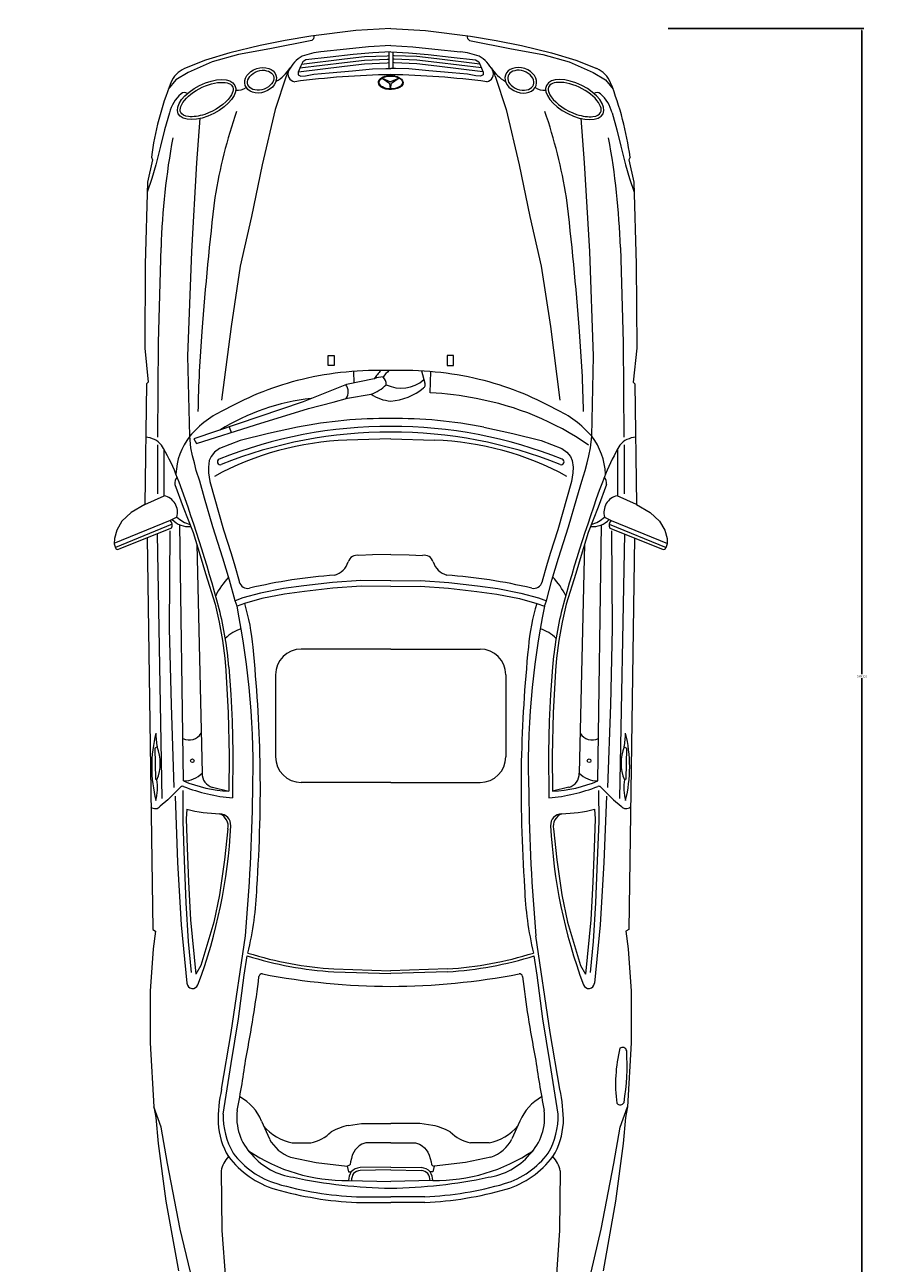
# Model space of a CAD drawing. Units: inches. Extents: x 2599 to 2953, y 557 to 1152.
# Tile 3 of 7: x 2794 to 2874, y 621 to 734. Entities that reach past the tile are written whole.
import ezdxf

# ---------------------------------------------------------------- set-up
doc = ezdxf.new("R2010")
doc.units = ezdxf.units.IN
doc.layers.add('0_Equip', color=250, linetype='Continuous', lineweight=13)
doc.layers.add('A-ANNO-DIMS', color=2, linetype='Continuous', lineweight=18)
doc.styles.get("Standard").update_dxf_attribs({"font": 'arial.ttf'})
doc.dimstyles.get("Standard").update_dxf_attribs({"dimtxt": 0.18, "dimasz": 0.18, "dimexe": 0.18, "dimexo": 0.0625, "dimgap": 0.09, "dimtad": 0, "dimtih": 1, "dimtoh": 1, "dimdec": 4, "dimzin": 0, "dimdsep": 46, "dimtxsty": 'Standard', "dimcen": 0.09, "dimadec": 0, "dimazin": 0, "dimtfac": 1, "dimtdec": 4, "dimtofl": 0, "dimtmove": 0, "dimatfit": 3, "dimfxl": 1, "dimtolj": 1, "dimtzin": 0, "dimarcsym": 0})

# ---------------------------------------------------------------- blocks, each defined once
blk = doc.blocks.new('A$C4C7B54D1')
at = {"layer": '0_Equip', "ltscale": 0.1}
for p, q in [((-0.7257, 2.678), (-0.8531, 2.6707)), ((-0.7257, 2.678), (-0.5983, 2.6707)), ((-1.112, 2.6343), (-1.2037, 2.6168)), ((-1.0138, 2.6343), (-1.1673, 2.6045)), ((-1.0176, 2.6505), (-1.112, 2.6343)), ((-0.8531, 2.6707), (-1.0176, 2.6505)), ((-0.5983, 2.6707), (-0.4338, 2.6505)), ((-0.4376, 2.6343), (-0.284, 2.6045)), ((-0.4338, 2.6505), (-0.3394, 2.6343)), ((-0.3394, 2.6343), (-0.2477, 2.6168)), ((-1.3142, 2.5898), (-1.4032, 2.5628)), ((-1.2824, 2.5829), (-1.3789, 2.557)), ((-1.2037, 2.6168), (-1.3142, 2.5898)), ((-1.1673, 2.6045), (-1.2824, 2.5829)), ((-0.8877, 2.6027), (-0.9812, 2.5937)), ((-0.8072, 2.6112), (-0.8877, 2.6027)), ((-0.7257, 2.6157), (-0.8072, 2.6112)), ((-0.7257, 2.6157), (-0.6441, 2.6112)), ((-0.6441, 2.6112), (-0.5636, 2.6027)), ((-0.5636, 2.6027), (-0.4701, 2.5937)), ((-0.284, 2.6045), (-0.1689, 2.5829)), ((-0.2477, 2.6168), (-0.1371, 2.5898)), ((-0.1689, 2.5829), (-0.0725, 2.557)), ((-0.1371, 2.5898), (-0.0481, 2.5628)), ((-1.4032, 2.5628), (-1.4801, 2.5318)), ((-1.3789, 2.557), (-1.4667, 2.5181)), ((-0.0725, 2.557), (0.0153, 2.5181)), ((-0.0481, 2.5628), (0.0288, 2.5318)), ((-1.4667, 2.5181), (-1.5113, 2.4907)), ((-1.1083, 2.5037), (-1.1486, 2.3827)), ((-0.343, 2.5037), (-0.3027, 2.3827)), ((0.0153, 2.5181), (0.06, 2.4907)), ((-1.5113, 2.4907), (-1.5393, 2.4562)), ((0.06, 2.4907), (0.0879, 2.4562)), ((-1.5353, 2.3701), (-1.5529, 2.308)), ((-1.1486, 2.3827), (-1.1961, 2.1797)), ((-0.3027, 2.3827), (-0.2552, 2.1797)), ((0.084, 2.3701), (0.1016, 2.308)), ((-1.435, 2.1869), (-1.4221, 2.3511)), ((-0.0163, 2.1869), (-0.0293, 2.3511)), ((-1.5529, 2.308), (-1.5677, 2.2486)), ((0.1016, 2.308), (0.1164, 2.2486)), ((-1.5677, 2.2486), (-1.5849, 2.1795)), ((0.1164, 2.2486), (0.1336, 2.1795)), ((-1.597, 2.1976), (-1.615, 2.1169)), ((-1.6012, 2.2082), (-1.597, 2.1976)), ((-1.5849, 2.1795), (-1.5997, 2.1304)), ((-1.4537, 1.863), (-1.435, 2.1869)), ((-1.1961, 2.1797), (-1.2349, 1.9911)), ((-0.2552, 2.1797), (-0.2164, 1.9911)), ((0.0024, 1.863), (-0.0163, 2.1869)), ((0.1336, 2.1795), (0.1484, 2.1304)), ((0.1499, 2.2082), (0.1457, 2.1976)), ((0.1457, 2.1976), (0.1637, 2.1169)), ((-1.5997, 2.1304), (-1.6161, 2.0798)), ((0.1484, 2.1304), (0.1647, 2.0798)), ((-1.615, 2.1169), (-1.6235, 1.8165)), ((0.1637, 2.1169), (0.1722, 1.8165)), ((-1.2349, 1.9911), (-1.2767, 1.8097)), ((-0.2164, 1.9911), (-0.1746, 1.8097)), ((-1.566, 1.8774), (-1.5761, 1.5304)), ((-1.4681, 1.48), (-1.4537, 1.863)), ((0.0168, 1.48), (0.0024, 1.863)), ((0.1147, 1.8774), (0.1247, 1.5304)), ((-1.6235, 1.8165), (-1.6256, 1.5098)), ((0.1722, 1.8165), (0.1743, 1.5098)), ((-1.2767, 1.8097), (-1.3098, 1.588)), ((-0.1746, 1.8097), (-0.1415, 1.588)), ((-1.3098, 1.588), (-1.3443, 1.3187)), ((-0.1415, 1.588), (-0.107, 1.3187)), ((-1.6256, 1.5098), (-1.6129, 1.3846)), ((-1.5761, 1.5304), (-1.5789, 1.1834)), ((0.1247, 1.5304), (0.1276, 1.1834)), ((0.1743, 1.5098), (0.1616, 1.3846)), ((-1.461, 1.1868), (-1.4681, 1.48)), ((-0.955, 1.4459), (-0.955, 1.4827)), ((-0.955, 1.4827), (-0.9321, 1.4827)), ((-0.9321, 1.4827), (-0.9321, 1.4459)), ((-0.5192, 1.4827), (-0.5192, 1.4459)), ((-0.4964, 1.4827), (-0.5192, 1.4827)), ((-0.4964, 1.4459), (-0.4964, 1.4827)), ((0.0097, 1.1868), (0.0168, 1.48)), ((-0.9321, 1.4459), (-0.955, 1.4459)), ((-0.8614, 1.4242), (-0.8603, 1.382)), ((-0.6135, 1.4258), (-0.6012, 1.3814)), ((-0.5809, 1.3459), (-0.5793, 1.4233)), ((-0.5192, 1.4459), (-0.4964, 1.4459)), ((-1.6193, 1.3782), (-1.6252, 0.9375)), ((-1.6129, 1.3846), (-1.6193, 1.3782)), ((-0.8878, 1.3764), (-1.0456, 1.313)), ((-0.7861, 1.3973), (-0.8878, 1.3764)), ((0.1616, 1.3846), (0.1679, 1.3782)), ((0.1679, 1.3782), (0.1739, 0.9375)), ((-0.9361, 1.3119), (-0.8835, 1.3269)), ((-0.8835, 1.3269), (-0.7975, 1.3408)), ((-1.0456, 1.313), (-1.4462, 1.1776)), ((-1.2207, 1.2292), (-1.0263, 1.2883)), ((-1.0263, 1.2883), (-0.9361, 1.3119)), ((-1.4366, 1.1604), (-1.2207, 1.2292)), ((-1.4565, 1.1447), (-1.461, 1.1868)), ((-1.3162, 1.2215), (-1.3088, 1.2011)), ((-1.1723, 1.1976), (-1.2762, 1.1716)), ((-1.0667, 1.22), (-1.1723, 1.1976)), ((-0.3847, 1.22), (-0.279, 1.1976)), ((-0.279, 1.1976), (-0.1751, 1.1716)), ((0.0052, 1.1447), (0.0097, 1.1868)), ((-1.5793, 1.1562), (-1.5793, 0.9761)), ((-1.5552, 1.139), (-1.5552, 0.9693)), ((-1.4503, 1.1151), (-1.4565, 1.1447)), ((-1.4462, 1.1776), (-1.4366, 1.1604)), ((-1.3515, 1.142), (-1.3703, 1.1286)), ((-1.2762, 1.1716), (-1.3515, 1.142)), ((-0.7257, 1.1776), (-0.8858, 1.1725)), ((-0.7257, 1.1776), (-0.5655, 1.1725)), ((-0.1751, 1.1716), (-0.0999, 1.142)), ((-0.0999, 1.142), (-0.0811, 1.1286)), ((-0.0011, 1.1151), (0.0052, 1.1447)), ((0.1038, 1.139), (0.1038, 0.9693)), ((0.128, 1.1562), (0.128, 0.9761)), ((-1.444, 1.0892), (-1.4503, 1.1151)), ((-1.4368, 1.0623), (-1.444, 1.0892)), ((-1.39, 1.0981), (-1.3927, 1.0739)), ((-1.3828, 1.1133), (-1.39, 1.0981)), ((-1.3703, 1.1286), (-1.3828, 1.1133)), ((-0.0811, 1.1286), (-0.0685, 1.1133)), ((-0.0685, 1.1133), (-0.0614, 1.0981)), ((-0.0614, 1.0981), (-0.0587, 1.0739)), ((-0.0145, 1.0623), (-0.0073, 1.0892)), ((-0.0073, 1.0892), (-0.0011, 1.1151)), ((-1.4243, 1.0229), (-1.4368, 1.0623)), ((-1.3927, 1.0739), (-1.3918, 1.0533)), ((-1.3918, 1.0533), (-1.3867, 1.0211)), ((-0.0596, 1.0533), (-0.0646, 1.0211)), ((-0.0587, 1.0739), (-0.0596, 1.0533)), ((-0.027, 1.0229), (-0.0145, 1.0623)), ((-1.5149, 1.011), (-1.4844, 0.9277)), ((-1.4064, 0.961), (-1.4243, 1.0229)), ((-1.3867, 1.0211), (-1.3374, 0.8446)), ((-0.0646, 1.0211), (-0.1139, 0.8446)), ((-0.0449, 0.961), (-0.027, 1.0229)), ((0.0635, 1.011), (0.0331, 0.9277)), ((-1.6252, 0.9375), (-1.5546, 0.9696)), ((-1.3759, 0.8562), (-1.4064, 0.961)), ((-0.0754, 0.8562), (-0.0449, 0.961)), ((0.1739, 0.9375), (0.1032, 0.9696)), ((-1.6745, 0.908), (-1.7088, 0.8764)), ((-1.6252, 0.9375), (-1.6745, 0.908)), ((-1.4844, 0.9277), (-1.4486, 0.8345)), ((0.0331, 0.9277), (-0.0028, 0.8345)), ((0.1739, 0.9375), (0.2232, 0.908)), ((0.2232, 0.908), (0.2574, 0.8764)), ((-1.5321, 0.8786), (-1.7381, 0.7945)), ((-1.5253, 0.865), (-1.7329, 0.7802)), ((-1.7088, 0.8764), (-1.728, 0.8432)), ((-1.508, 0.8914), (-1.5321, 0.8786)), ((-1.4835, -0.0735), (-1.497, 0.863)), ((0.0322, -0.0735), (0.0457, 0.863)), ((0.0566, 0.8914), (0.0807, 0.8786)), ((0.074, 0.865), (0.2816, 0.7802)), ((0.0807, 0.8786), (0.2867, 0.7945)), ((0.2574, 0.8764), (0.2767, 0.8432)), ((-1.728, 0.8432), (-1.7366, 0.8127)), ((-1.5273, 0.8512), (-1.7203, 0.7738)), ((-1.5805, 0.8299), (-1.5623, -0.138)), ((-1.5337, 0.8406), (-1.5355, 0.484)), ((-1.4486, 0.8345), (-1.4226, 0.7503)), ((-1.3401, 0.7406), (-1.3759, 0.8562)), ((-1.3374, 0.8446), (-1.3097, 0.7577)), ((-0.1139, 0.8446), (-0.1417, 0.7577)), ((-0.1112, 0.7406), (-0.0754, 0.8562)), ((-0.0028, 0.8345), (-0.0287, 0.7503)), ((0.0759, 0.8512), (0.269, 0.7738)), ((0.0824, 0.8406), (0.0842, 0.484)), ((0.1292, 0.8299), (0.111, -0.138)), ((0.2767, 0.8432), (0.2853, 0.8127)), ((-1.7366, 0.8127), (-1.7377, 0.7934)), ((-1.7377, 0.7934), (-1.7327, 0.7794)), ((-1.6171, 0.8152), (-1.5964, -0.6171)), ((-1.4352, 0.792), (-1.4152, -0.045)), ((-0.0162, 0.792), (-0.0361, -0.045)), ((0.1658, 0.8152), (0.145, -0.6171)), ((0.2863, 0.7934), (0.2813, 0.7794)), ((0.2853, 0.8127), (0.2863, 0.7934)), ((-1.4226, 0.7503), (-1.4029, 0.6849)), ((-1.315, 0.66), (-1.3401, 0.7406)), ((-1.3097, 0.7577), (-1.2953, 0.7129)), ((-0.7926, 0.7532), (-0.8418, 0.7514)), ((-0.7257, 0.7541), (-0.7926, 0.7532)), ((-0.7257, 0.7541), (-0.6587, 0.7532)), ((-0.6587, 0.7532), (-0.6095, 0.7514)), ((-0.1417, 0.7577), (-0.156, 0.7129)), ((-0.1363, 0.66), (-0.1112, 0.7406)), ((-0.0287, 0.7503), (-0.0484, 0.6849)), ((-1.4029, 0.6849), (-1.368, 0.5729)), ((-1.2953, 0.7129), (-1.2801, 0.6573)), ((-0.156, 0.7129), (-0.1712, 0.6573)), ((-0.0484, 0.6849), (-0.0834, 0.5729)), ((-1.2951, 0.5849), (-1.315, 0.66)), ((-1.2801, 0.6573), (-1.2795, 0.6546)), ((-1.0437, 0.6403), (-1.1177, 0.6302)), ((-0.9389, 0.6526), (-1.0437, 0.6403)), ((-0.8346, 0.6593), (-0.9389, 0.6526)), ((-0.834, 0.6384), (-0.937, 0.6317)), ((-0.7257, 0.6582), (-0.8346, 0.6593)), ((-0.7257, 0.6373), (-0.834, 0.6384)), ((-0.7257, 0.6582), (-0.6168, 0.6593)), ((-0.7257, 0.6373), (-0.6173, 0.6384)), ((-0.6173, 0.6384), (-0.5143, 0.6317)), ((-0.6168, 0.6593), (-0.5124, 0.6526)), ((-0.5124, 0.6526), (-0.4076, 0.6403)), ((-0.4076, 0.6403), (-0.3337, 0.6302)), ((-0.1712, 0.6573), (-0.1719, 0.6546)), ((-0.1562, 0.5849), (-0.1363, 0.66)), ((-1.2663, 0.5956), (-1.2951, 0.5849)), ((-1.2021, 0.6133), (-1.2663, 0.5956)), ((-1.1973, 0.593), (-1.2599, 0.5757)), ((-1.1177, 0.6302), (-1.2021, 0.6133)), ((-1.1142, 0.6096), (-1.1973, 0.593)), ((-1.0411, 0.6196), (-1.1142, 0.6096)), ((-0.937, 0.6317), (-1.0411, 0.6196)), ((-0.5143, 0.6317), (-0.4102, 0.6196)), ((-0.4102, 0.6196), (-0.3371, 0.6096)), ((-0.3371, 0.6096), (-0.2541, 0.593)), ((-0.3337, 0.6302), (-0.2492, 0.6133)), ((-0.2541, 0.593), (-0.1914, 0.5757)), ((-0.2492, 0.6133), (-0.185, 0.5956)), ((-0.185, 0.5956), (-0.1562, 0.5849)), ((-1.368, 0.5729), (-1.3527, 0.5066)), ((-1.2879, 0.5653), (-1.2951, 0.5849)), ((-1.2599, 0.5757), (-1.2879, 0.5653)), ((-0.1914, 0.5757), (-0.1635, 0.5653)), ((-0.1635, 0.5653), (-0.1562, 0.5849)), ((-0.0834, 0.5729), (-0.0986, 0.5066)), ((-1.3527, 0.5066), (-1.3411, 0.4394)), ((-0.0986, 0.5066), (-0.1102, 0.4394)), ((-1.5355, 0.484), (-1.5292, 0.2045)), ((0.0842, 0.484), (0.0779, 0.2045)), ((-1.3411, 0.4394), (-1.3321, 0.3749)), ((-0.7257, 0.4085), (-1.0528, 0.4085)), ((-0.7257, 0.4085), (-0.3986, 0.4085)), ((-0.1102, 0.4394), (-0.1192, 0.3749)), ((-1.3321, 0.3749), (-1.3286, 0.3301)), ((-0.1192, 0.3749), (-0.1228, 0.3301)), ((-1.3286, 0.3301), (-1.3204, 0.1751)), ((-1.3178, 0.3418), (-1.31, 0.2426)), ((-0.1335, 0.3418), (-0.1413, 0.2426)), ((-0.1228, 0.3301), (-0.1309, 0.1751)), ((-1.1468, 0.3145), (-1.1468, 0.0145)), ((-0.3045, 0.3145), (-0.3045, 0.0145)), ((-1.31, 0.2426), (-1.306, 0.1454)), ((-0.1413, 0.2426), (-0.1454, 0.1454)), ((-1.5292, 0.2045), (-1.5185, -0.0974)), ((0.0779, 0.2045), (0.0672, -0.0974)), ((-1.3204, 0.1751), (-1.3164, 0.0193)), ((-1.306, 0.1454), (-1.3036, 0.0305)), ((-0.1454, 0.1454), (-0.1478, 0.0305)), ((-0.1309, 0.1751), (-0.1349, 0.0193)), ((-1.5798, 0.0505), (-1.5879, 0.0456)), ((-1.5879, 0.0456), (-1.5863, -0.0676)), ((0.1285, 0.0505), (0.1365, 0.0456)), ((0.1365, 0.0456), (0.1349, -0.0676)), ((-1.3164, 0.0193), (-1.3178, -0.1112)), ((-1.3036, 0.0305), (-1.3044, -0.1358)), ((-0.1478, 0.0305), (-0.147, -0.1358)), ((-0.1349, 0.0193), (-0.1335, -0.1112)), ((-1.5863, -0.0676), (-1.5806, -0.0692)), ((-0.7257, -0.0796), (-1.0528, -0.0796)), ((-0.7257, -0.0796), (-0.3986, -0.0796)), ((0.1349, -0.0676), (0.1293, -0.0692)), ((-1.4948, -0.0965), (-1.5413, -0.143)), ((-1.5147, -0.1299), (-1.5058, -0.3725)), ((-1.4857, -0.1082), (-1.4866, -0.2223)), ((-1.3774, -0.0972), (-1.3178, -0.1112)), ((-0.0739, -0.0972), (-0.1335, -0.1112)), ((0.0344, -0.1082), (0.0352, -0.2223)), ((0.0435, -0.0965), (0.0899, -0.143)), ((0.0633, -0.1299), (0.0545, -0.3725)), ((-1.5413, -0.143), (-1.5686, -0.1663)), ((-1.4713, -0.1773), (-1.4737, -0.2127)), ((0.02, -0.1773), (0.0224, -0.2127)), ((0.0899, -0.143), (0.1172, -0.1663)), ((-1.4866, -0.2223), (-1.4809, -0.3653)), ((-1.4737, -0.2127), (-1.4705, -0.3187)), ((0.0224, -0.2127), (0.0192, -0.3187)), ((0.0352, -0.2223), (0.0296, -0.3653)), ((-1.3211, -0.2496), (-1.3332, -0.3629)), ((-0.1302, -0.2496), (-0.1182, -0.3629)), ((-1.4705, -0.3187), (-1.4649, -0.4424)), ((0.0192, -0.3187), (0.0135, -0.4424)), ((-1.5058, -0.3725), (-1.4922, -0.6007)), ((-1.4809, -0.3653), (-1.4745, -0.5203)), ((-1.3332, -0.3629), (-1.3516, -0.4906)), ((-0.1182, -0.3629), (-0.0997, -0.4906)), ((0.0296, -0.3653), (0.0232, -0.5203)), ((0.0545, -0.3725), (0.0408, -0.6007)), ((-1.4649, -0.4424), (-1.4576, -0.5822)), ((0.0135, -0.4424), (0.0063, -0.5822)), ((-1.3516, -0.4906), (-1.3725, -0.5902)), ((-0.0997, -0.4906), (-0.0788, -0.5902)), ((-1.4745, -0.5203), (-1.4665, -0.6617)), ((0.0232, -0.5203), (0.0151, -0.6617)), ((-1.4576, -0.5822), (-1.4384, -0.7806)), ((0.0063, -0.5822), (-0.013, -0.7806)), ((-1.5964, -0.6171), (-1.5863, -0.6228)), ((-1.5863, -0.6228), (-1.5949, -0.6885)), ((-1.4922, -0.6007), (-1.4712, -0.814)), ((-1.3725, -0.5902), (-1.3942, -0.6641)), ((-0.0788, -0.5902), (-0.0571, -0.6641)), ((0.0408, -0.6007), (0.0198, -0.814)), ((0.145, -0.6171), (0.1349, -0.6228)), ((0.1349, -0.6228), (0.1436, -0.6885)), ((-1.4665, -0.6617), (-1.4552, -0.7742)), ((-1.3942, -0.6641), (-1.4199, -0.7485)), ((-1.3094, -0.9936), (-1.2569, -0.6398)), ((-0.1419, -0.9936), (-0.1944, -0.6398)), ((-0.0571, -0.6641), (-0.0314, -0.7485)), ((0.0151, -0.6617), (0.0039, -0.7742)), ((-1.5949, -0.6885), (-1.605, -0.843)), ((-1.2616, -0.7846), (-1.2511, -0.7134)), ((-0.1898, -0.7846), (-0.2003, -0.7134)), ((0.1436, -0.6885), (0.1537, -0.843)), ((-1.4199, -0.7485), (-1.4384, -0.7806)), ((-0.9331, -0.7613), (-0.7253, -0.7683)), ((-0.5182, -0.7613), (-0.726, -0.7683)), ((-0.0314, -0.7485), (-0.013, -0.7806)), ((-1.2826, -0.9445), (-1.2616, -0.7846)), ((-0.9336, -0.7717), (-0.7257, -0.7787)), ((-0.5177, -0.7717), (-0.7257, -0.7787)), ((-0.1688, -0.9445), (-0.1898, -0.7846)), ((-1.605, -0.843), (-1.605, -1.0322)), ((0.1537, -0.843), (0.1537, -1.0322)), ((-1.3094, -1.1068), (-1.2826, -0.9445)), ((-0.1419, -1.1068), (-0.1688, -0.9445)), ((-1.3444, -1.2014), (-1.3094, -0.9936)), ((-0.1069, -1.2014), (-0.1419, -0.9936)), ((-1.605, -1.0322), (-1.592, -1.2661)), ((0.1537, -1.0322), (0.1407, -1.2661)), ((-1.3386, -1.2925), (-1.3094, -1.1068)), ((-0.1127, -1.2925), (-0.1419, -1.1068)), ((-1.565, -1.3405), (-1.592, -1.2661)), ((-1.592, -1.2661), (-1.5848, -1.3051)), ((0.1137, -1.3405), (0.1407, -1.2661)), ((0.1407, -1.2661), (0.1335, -1.3051)), ((-1.5848, -1.3051), (-1.5762, -1.4004)), ((0.1335, -1.3051), (0.1248, -1.4004)), ((-1.5417, -1.4736), (-1.565, -1.3405)), ((-1.1985, -1.3182), (-1.1694, -1.3835)), ((-0.88, -1.3337), (-0.8328, -1.3271)), ((-0.8328, -1.3271), (-0.7257, -1.3271)), ((-0.6185, -1.3271), (-0.7257, -1.3271)), ((-0.5713, -1.3337), (-0.6185, -1.3271)), ((-0.2528, -1.3182), (-0.282, -1.3835)), ((0.0904, -1.4736), (0.1137, -1.3405)), ((-1.5762, -1.4004), (-1.5486, -1.6107)), ((-1.0858, -1.3979), (-1.0181, -1.3979)), ((-0.8309, -1.402), (-0.8409, -1.4088)), ((-0.8163, -1.3979), (-0.8309, -1.402)), ((-0.7257, -1.3974), (-0.8163, -1.3979)), ((-0.7257, -1.3974), (-0.635, -1.3979)), ((-0.635, -1.3979), (-0.6204, -1.402)), ((-0.6204, -1.402), (-0.6104, -1.4088)), ((-0.3655, -1.3979), (-0.4333, -1.3979)), ((0.1248, -1.4004), (0.0973, -1.6107)), ((-0.8664, -1.4423), (-0.8696, -1.4545)), ((-0.861, -1.4312), (-0.8664, -1.4423)), ((-0.8558, -1.4236), (-0.861, -1.4312)), ((-0.8488, -1.4158), (-0.8558, -1.4236)), ((-0.8409, -1.4088), (-0.8488, -1.4158)), ((-0.6104, -1.4088), (-0.6025, -1.4158)), ((-0.6025, -1.4158), (-0.5955, -1.4236)), ((-0.5955, -1.4236), (-0.5904, -1.4312)), ((-0.5904, -1.4312), (-0.585, -1.4423)), ((-0.585, -1.4423), (-0.5817, -1.4545)), ((-1.4962, -1.7129), (-1.5417, -1.4736)), ((-1.0923, -1.4501), (-0.9989, -1.4699)), ((-0.9989, -1.4699), (-0.8846, -1.4828)), ((-0.8807, -1.4821), (-0.8846, -1.4828)), ((-0.8846, -1.4828), (-0.8799, -1.5038)), ((-0.8769, -1.4791), (-0.8807, -1.4821)), ((-0.8745, -1.477), (-0.8769, -1.4791)), ((-0.8731, -1.467), (-0.8745, -1.477)), ((-0.8696, -1.4545), (-0.8731, -1.467)), ((-0.7257, -1.4865), (-0.8374, -1.4884)), ((-0.7257, -1.4865), (-0.6139, -1.4884)), ((-0.5817, -1.4545), (-0.5782, -1.467)), ((-0.5782, -1.467), (-0.5768, -1.477)), ((-0.5768, -1.477), (-0.5744, -1.4791)), ((-0.5744, -1.4791), (-0.5706, -1.4821)), ((-0.5668, -1.4828), (-0.5714, -1.5038)), ((-0.5706, -1.4821), (-0.5668, -1.4828)), ((-0.4524, -1.4699), (-0.5668, -1.4828)), ((-0.359, -1.4501), (-0.4524, -1.4699)), ((0.0448, -1.7129), (0.0904, -1.4736)), ((-1.3456, -1.5004), (-1.3433, -1.7188)), ((-0.8799, -1.5038), (-0.8706, -1.5038)), ((-0.8799, -1.5352), (-0.7257, -1.5393)), ((-0.7257, -1.4969), (-0.837, -1.4988)), ((-0.7257, -1.4969), (-0.6143, -1.4988)), ((-0.5714, -1.5352), (-0.7257, -1.5393)), ((-0.5714, -1.5038), (-0.5808, -1.5038)), ((-0.1057, -1.5004), (-0.1081, -1.7188)), ((-1.5486, -1.6107), (-1.5024, -1.8663)), ((-0.8507, -1.616), (-0.7257, -1.616)), ((-0.8502, -1.5951), (-0.7257, -1.5951)), ((-0.6011, -1.5951), (-0.7257, -1.5951)), ((-0.6006, -1.616), (-0.7257, -1.616)), ((0.0973, -1.6107), (0.0511, -1.8663)), ((-1.4584, -1.8701), (-1.4962, -1.7129)), ((-1.3433, -1.7188), (-1.3304, -1.8962)), ((-0.1081, -1.7188), (-0.1209, -1.8962)), ((0.0071, -1.8701), (0.0448, -1.7129))]:
    blk.add_line(p, q, dxfattribs=at)
at = {"layer": '0_Equip'}
for p, q in [((-0.8628, 2.5838), (-0.9467, 2.5739)), ((-0.7905, 2.5897), (-0.8628, 2.5838)), ((-0.7257, 2.5926), (-0.7905, 2.5897)), ((-0.733, 2.5923), (-0.733, 2.5325)), ((-0.7257, 2.5926), (-0.6608, 2.5897)), ((-0.7183, 2.5923), (-0.7183, 2.5325)), ((-0.6608, 2.5897), (-0.5886, 2.5838)), ((-0.5886, 2.5838), (-0.5046, 2.5739)), ((-1.0545, 2.5425), (-1.0638, 2.5185)), ((-1.0631, 2.5204), (-0.8949, 2.5405)), ((-1.0577, 2.5343), (-0.8949, 2.5537)), ((-1.0475, 2.557), (-1.0545, 2.5425)), ((-1.0517, 2.5482), (-0.8949, 2.567)), ((-1.0364, 2.5634), (-1.0475, 2.557)), ((-0.9467, 2.5739), (-1.0364, 2.5634)), ((-0.8949, 2.567), (-0.8211, 2.5763)), ((-0.8949, 2.5537), (-0.8211, 2.5631)), ((-0.8949, 2.5405), (-0.8211, 2.5498)), ((-0.8211, 2.5763), (-0.738, 2.5791)), ((-0.8211, 2.5631), (-0.738, 2.5659)), ((-0.8211, 2.5498), (-0.738, 2.5526)), ((-0.738, 2.5791), (-0.733, 2.58)), ((-0.738, 2.5659), (-0.733, 2.5668)), ((-0.738, 2.5526), (-0.733, 2.5536)), ((-0.7133, 2.5791), (-0.7183, 2.58)), ((-0.7133, 2.5659), (-0.7183, 2.5668)), ((-0.7133, 2.5526), (-0.7183, 2.5536)), ((-0.6302, 2.5763), (-0.7133, 2.5791)), ((-0.6302, 2.5631), (-0.7133, 2.5659)), ((-0.6302, 2.5498), (-0.7133, 2.5526)), ((-0.5564, 2.567), (-0.6302, 2.5763)), ((-0.5564, 2.5537), (-0.6302, 2.5631)), ((-0.5564, 2.5405), (-0.6302, 2.5498)), ((-0.3996, 2.5482), (-0.5564, 2.567)), ((-0.3936, 2.5343), (-0.5564, 2.5537)), ((-0.3882, 2.5204), (-0.5564, 2.5405)), ((-0.5046, 2.5739), (-0.4149, 2.5634)), ((-0.4149, 2.5634), (-0.4038, 2.557)), ((-0.4038, 2.557), (-0.3968, 2.5425)), ((-0.3968, 2.5425), (-0.3875, 2.5185)), ((-1.0638, 2.5185), (-1.0638, 2.5092)), ((-1.0638, 2.5092), (-1.0545, 2.504)), ((-1.0545, 2.504), (-1.0376, 2.5051)), ((-1.0376, 2.5051), (-1.0067, 2.5116)), ((-1.0067, 2.5116), (-0.9502, 2.5168)), ((-0.9502, 2.5168), (-0.8657, 2.5238)), ((-0.8657, 2.5238), (-0.7922, 2.5308)), ((-0.7922, 2.5308), (-0.7433, 2.5325)), ((-0.7566, 2.4971), (-0.7261, 2.4828)), ((-0.7566, 2.4971), (-0.7291, 2.4776)), ((-0.7433, 2.5325), (-0.7257, 2.5325)), ((-0.7389, 2.5095), (-0.7395, 2.5059)), ((-0.6947, 2.4974), (-0.7261, 2.4828)), ((-0.708, 2.5325), (-0.7257, 2.5325)), ((-0.6947, 2.4974), (-0.723, 2.4776)), ((-0.7124, 2.5095), (-0.7119, 2.5059)), ((-0.6591, 2.5308), (-0.708, 2.5325)), ((-0.5857, 2.5238), (-0.6591, 2.5308)), ((-0.5011, 2.5168), (-0.5857, 2.5238)), ((-0.4446, 2.5116), (-0.5011, 2.5168)), ((-0.4137, 2.5051), (-0.4446, 2.5116)), ((-0.3968, 2.504), (-0.4137, 2.5051)), ((-0.3875, 2.5092), (-0.3968, 2.504)), ((-0.3875, 2.5185), (-0.3875, 2.5092)), ((-0.7259, 2.4578), (-0.7291, 2.4776)), ((-0.7259, 2.4578), (-0.723, 2.4776))]:
    blk.add_line(p, q, dxfattribs=at)
at = {"layer": '0_Equip', "ltscale": 0.1}
for centre in [(-1.4513, 0), (0, 0)]:
    blk.add_circle(centre, 0.00662, dxfattribs=at)
for centre, radius, start, end in [((-1.0252, 2.6508), 0.02, 304.7228, 3.5172), ((-0.4261, 2.6508), 0.02, 176.4828, 235.2772), ((-0.9299, 2.2354), 0.3619, 98.1466, 109.2524), ((-0.5214, 2.2354), 0.3619, 70.7476, 81.8534), ((-0.9799, 2.461), 0.1353, 120.8369, 151.2853), ((-0.4714, 2.461), 0.1353, 28.7147, 59.1631), ((-1.4391, 2.4422), 0.0986, 114.5945, 157.5113), ((-1.2153, 2.6098), 0.1432, 299.1564, 328.1831), ((-0.9799, 2.461), 0.1353, 151.2853, 161.5889), ((-1.0728, 2.5126), 0.029, 152.6038, 261.721), ((-0.6679, -0.6671), 3.1773, 91.0415, 97.3969), ((-0.7834, -0.6671), 3.1773, 82.6031, 88.9585), ((-0.3785, 2.5126), 0.029, 278.279, 27.3962), ((-0.236, 2.6098), 0.1432, 211.8169, 240.8436), ((-0.4714, 2.461), 0.1353, 18.4111, 28.7147), ((-0.0123, 2.4422), 0.0986, 22.4887, 65.4055), ((-0.4722, 2.0579), 1.139, 158.2564, 172.4203), ((-1.2841, 2.5028), 0.0501, 260.5448, 306.7068), ((-0.1672, 2.5028), 0.0501, 233.2932, 279.4552), ((-0.9791, 2.0579), 1.139, 7.5797, 21.7436), ((-1.4083, 2.3394), 0.1306, 130.2084, 166.4224), ((-1.4798, 2.4259), 0.0184, 54.8052, 134.0204), ((0.0285, 2.4259), 0.0184, 45.9796, 125.1948), ((-0.043, 2.3394), 0.1306, 13.5776, 49.7916), ((0.5502, 1.746), 1.9445, 161.1117, 170.7019), ((-2.0015, 1.746), 1.9445, 9.2981, 18.8883), ((1.1202, 1.7918), 2.6875, 169.5541, 178.1755), ((-2.5715, 1.7918), 2.6875, 1.8245, 10.4459), ((9.2655, 0.7813), 10.7109, 173.14258, 175.77374), ((-10.7169, 0.7813), 10.7109, 4.22626, 6.85742), ((2.9623, 1.2089), 4.3935, 175.2767, 179.1124), ((-4.4136, 1.2089), 4.3935, 0.8876, 4.7233), ((-0.7686, 0.201), 1.2267, 87.9955, 103.2364), ((-0.3726, 1.0935), 0.5131, 139.3585, 143.6922), ((-0.6528, 1.3354), 0.1211, 130.7679, 145.6911), ((-0.6828, 0.201), 1.2267, 76.7636, 92.0045), ((-0.786, 0.3109), 1.1158, 103.6551, 119.1148), ((-0.9216, 1.3498), 0.0409, 323.4512, 39.0343), ((-0.8494, 1.486), 0.1542, 289.6676, 314.192), ((-0.7554, 1.327), 0.0768, 88.1186, 113.6019), ((-0.7803, 1.3768), 0.0384, 357.9275, 44.3829), ((-0.6872, 1.4869), 0.1241, 243.8649, 311.6638), ((-0.741, 1.5272), 0.212, 274.1513, 309.4931), ((-0.6113, 1.3746), 0.0122, 294.8678, 33.6398), ((-0.6653, 0.3109), 1.1158, 60.8852, 76.3449), ((-0.929, 0.5266), 0.803, 96.22, 121.6991), ((-0.7147, 1.4628), 0.1474, 235.8143, 265.7174), ((-0.617, 0.3882), 0.9584, 77.6919, 87.8428), ((-0.5976, 0.2949), 1.0461, 55.3038, 79.8165), ((-1.1803, 0.9494), 0.3676, 113.8511, 139.7847), ((-0.2711, 0.9494), 0.3676, 40.2153, 66.1489), ((-0.7478, -0.378), 1.6295, 89.2231, 101.2856), ((-0.7036, -0.378), 1.6295, 78.7144, 90.7769), ((-1.6261, 1.102), 0.0813, 40.278, 87.0689), ((-1.2706, 1.0395), 0.2408, 142.2718, 177.7746), ((-0.7356, -0.4312), 1.6538, 89.6554, 111.9286), ((-0.7356, -0.4312), 1.6329, 89.6554, 111.9286), ((-0.7157, -0.4312), 1.6538, 68.0714, 90.3446), ((-0.7157, -0.4312), 1.6329, 68.0714, 90.3446), ((-0.1807, 1.0395), 0.2408, 2.2254, 37.7282), ((0.1747, 1.102), 0.0813, 92.9311, 139.722), ((-2.3477, 0.6968), 0.9076, 22.824, 30.2904), ((-0.85, 0.0855), 1.0875, 91.8892, 118.6013), ((-0.6014, 0.0855), 1.0875, 61.3987, 88.1108), ((0.8964, 0.6968), 0.9076, 149.7096, 157.176), ((-1.3493, 1.0932), 0.0105, 111.9286, 291.9286), ((-0.102, 1.0932), 0.0105, 248.0714, 68.0714), ((-6.6059, -0.8606), 5.4408, 15.0904, 20.5451), ((5.1546, -0.8606), 5.4408, 159.4549, 164.9096), ((-1.4887, 1.0171), 0.0269, 132.3277, 193.1064), ((0.0373, 1.0171), 0.0269, 346.8936, 47.6723), ((-1.5684, 0.9084), 0.0628, 344.3283, 77.2348), ((0.1171, 0.9084), 0.0628, 102.7652, 195.6717), ((-1.5495, 0.8614), 0.0245, 335.4987, 44.5114), ((-1.463, 0.9441), 0.0879, 224.7932, 273.9292), ((-1.4233, 0.9849), 0.1262, 227.8287, 253.081), ((0.0117, 0.9441), 0.0879, 266.0708, 315.2068), ((-0.0281, 0.9849), 0.1262, 286.919, 312.1713), ((0.0982, 0.8614), 0.0245, 135.4886, 204.5013), ((-1.7238, 0.7825), 0.00941, 199.646, 291.8616), ((0.2725, 0.7825), 0.00941, 248.1384, 340.354), ((-0.9515, 0.7495), 0.0737, 286.567, 342.4011), ((-0.8474, 0.7163), 0.0355, 80.937, 162.15), ((-0.6039, 0.7163), 0.0355, 17.85, 99.063), ((-0.4998, 0.7495), 0.0737, 197.5989, 253.433), ((-1.1535, 0.5061), 0.2334, 134.9877, 155.4049), ((-1.249, 0.662), 0.0314, 193.667, 283.2045), ((-0.7896, -1.2957), 1.9795, 94.0807, 103.2045), ((-0.6617, -1.2957), 1.9795, 76.7955, 85.9193), ((-0.2023, 0.662), 0.0314, 256.7955, 346.333), ((-0.2978, 0.5061), 0.2334, 24.5951, 45.0123), ((-2.6334, 0.2371), 1.3197, 4.5498, 13.9797), ((-4.2099, -0.0242), 2.9809, 358.1905, 11.4064), ((-2.0025, 0.3511), 0.7759, 4.7259, 16.8296), ((2.7585, -0.0242), 2.9809, 168.5936, 181.8095), ((0.5512, 0.3511), 0.7759, 163.1704, 175.2741), ((1.1821, 0.2371), 1.3197, 166.0203, 175.4502), ((-1.2324, 0.3484), 0.1397, 106.6168, 134.6647), ((-0.2189, 0.3484), 0.1397, 45.3353, 73.3832), ((-6.5594, -0.126), 5.3575, 1.3159, 5.7952), ((-1.0528, 0.3145), 0.0941, 90, 180), ((-0.3986, 0.3145), 0.0941, 0, 90), ((5.1081, -0.126), 5.3575, 174.2048, 178.6841), ((-1.0944, -0.0222), 0.5055, 165.8807, 194.1193), ((-1.3066, 0.102), 0.2781, 180.1936, 190.6834), ((-1.4634, 0.1296), 0.0534, 245.2796, 326.9469), ((0.0121, 0.1296), 0.0534, 213.0531, 294.7204), ((-0.1448, 0.102), 0.2781, 349.3166, 359.8064), ((-0.3569, -0.0222), 0.5055, 345.8807, 14.1193), ((-1.7275, -0.0084), 0.159, 337.4976, 21.7335), ((0.2762, -0.0084), 0.159, 158.2665, 202.5024), ((-1.0528, 0.0145), 0.0941, 180, 270), ((-0.3986, 0.0145), 0.0941, 270, 0), ((-1.4831, 0.0214), 0.095, 269.7172, 315.6185), ((-1.3634, -0.0473), 0.0519, 177.4537, 254.2676), ((-6.573, -0.0941), 5.3705, 356.0501, 0.9723), ((5.1217, -0.0941), 5.3705, 179.0277, 183.9499), ((-0.0879, -0.0473), 0.0519, 285.7324, 2.5463), ((0.0317, 0.0214), 0.095, 224.3815, 270.2828), ((-1.7817, -0.0969), 0.2029, 346.1346, 7.8419), ((-1.2968, 0.3651), 0.4767, 246.9385, 267.4714), ((-0.1545, 0.3651), 0.4767, 272.5286, 293.0615), ((0.3303, -0.0969), 0.2029, 172.1581, 193.8654), ((-1.4874, -0.1039), 0.0105, 68.8598, 135.0096), ((-1.2476, 0.5164), 0.6547, 248.8598, 265.0222), ((-8.0298, -0.0355), 6.7998, 354.90123, 359.30214), ((6.5785, -0.0355), 6.7998, 180.69786, 185.09877), ((-0.2038, 0.5164), 0.6547, 274.9778, 291.1402), ((0.0361, -0.1039), 0.0105, 44.9904, 111.1402), ((-1.5869, -0.1514), 0.0236, 227.2909, 320.7388), ((-1.3362, 0.3542), 0.5484, 255.7347, 268.4072), ((-0.1152, 0.3542), 0.5484, 271.5928, 284.2653), ((0.1355, -0.1514), 0.0236, 219.2612, 312.7091), ((-1.3699, -0.2402), 0.0497, 349.0381, 68.1064), ((-1.3526, -0.2358), 0.0418, 357.143, 88.4072), ((-0.0988, -0.2358), 0.0418, 91.5928, 182.857), ((-0.0814, -0.2402), 0.0497, 111.8936, 190.9619), ((-3.2483, -0.1412), 1.9399, 339.54, 357.143), ((1.797, -0.1412), 1.9399, 182.857, 200.46), ((-2.454, -0.4173), 1.2396, 346.6558, 357.8401), ((1.0027, -0.4173), 1.2396, 182.1599, 193.3442), ((-0.8588, 0.5276), 1.3014, 252.4566, 266.7043), ((-0.8588, 0.5276), 1.291, 252.4566, 266.6988), ((-0.5926, 0.5276), 1.291, 273.3012, 287.5434), ((-0.5926, 0.5276), 1.3014, 273.2957, 287.5434), ((-1.4504, -0.812), 0.0209, 185.6259, 339.54), ((-5.088, -0.3237), 3.9082, 348.7726, 353.1671), ((-1.1971, -0.7899), 0.0105, 79.1189, 173.1671), ((-0.7142, 1.7227), 2.5481, 259.1189, 269.7413), ((-0.7372, 1.7227), 2.5481, 270.2587, 280.8811), ((-0.2542, -0.7899), 0.0105, 6.8329, 100.8811), ((3.6366, -0.3237), 3.9082, 186.8329, 191.2274), ((-0.001, -0.812), 0.0209, 200.46, 354.3741), ((-4.7286, -0.6026), 3.5073, 348.8701, 352.1003), ((3.2772, -0.6026), 3.5073, 187.8997, 191.1299), ((0.625, -1.1812), 0.5281, 165.7822, 187.813), ((0.1224, -1.0639), 0.0155, 11.61, 127.0083), ((-0.7003, -1.1122), 0.8395, 350.5693, 3.5107), ((-0.8187, -1.3185), 0.5386, 167.4447, 180.7102), ((-0.6326, -1.3185), 0.5386, 359.2898, 12.5553), ((-1.3591, -1.3822), 0.1728, 21.7432, 61.9432), ((-0.0922, -1.3822), 0.1728, 118.0568, 158.2568), ((0.1138, -1.243), 0.0156, 219.7819, 334.4738), ((-1.0611, -1.2979), 0.2775, 178.8811, 209.7062), ((-1.0952, -1.3051), 0.1937, 172.4314, 224.4267), ((-0.3561, -1.3051), 0.1937, 315.5733, 7.5686), ((-0.3902, -1.2979), 0.2775, 330.2938, 1.1189), ((-1.0944, -1.3104), 0.2633, 183.2136, 211.504), ((-1.0482, -1.2146), 0.1871, 220.4031, 258.3959), ((-1.0495, -1.2507), 0.1505, 282.0448, 314.7653), ((-0.8301, -1.5634), 0.235, 102.268, 118.8572), ((-0.6213, -1.5634), 0.235, 61.1428, 77.732), ((-0.4019, -1.2507), 0.1505, 225.2347, 257.9552), ((-0.4032, -1.2146), 0.1871, 281.6041, 319.5969), ((-0.3569, -1.3104), 0.2633, 328.496, 356.7864), ((-1.0421, -1.3141), 0.145, 208.6187, 249.7318), ((-0.4092, -1.3141), 0.145, 290.2682, 331.3813), ((-1.2501, -1.516), 0.0967, 135.2951, 170.7274), ((-1.052, -1.2472), 0.3339, 216.9484, 253.2314), ((-1.052, -1.2472), 0.313, 216.9484, 253.2054), ((-0.8912, -0.9022), 0.6331, 235.8724, 271.0227), ((-1.0459, -1.2776), 0.2487, 221.0065, 261.6946), ((-0.5601, -0.9022), 0.6331, 268.9773, 304.1276), ((-0.4054, -1.2776), 0.2487, 278.3054, 318.9935), ((-0.3993, -1.2472), 0.313, 286.7946, 323.0516), ((-0.3993, -1.2472), 0.3339, 286.7686, 323.0516), ((-0.2012, -1.516), 0.0967, 9.2726, 44.7049), ((-0.8344, -1.538), 0.0498, 93.4455, 136.5439), ((-0.6169, -1.538), 0.0498, 43.4561, 86.5545), ((-0.7003, 0.2815), 1.8451, 258.0669, 269.2129), ((-0.8066, -1.54), 0.0735, 150.5285, 176.2825), ((-0.8066, -1.54), 0.063, 151.7195, 175.9212), ((-0.8344, -1.538), 0.0393, 93.7549, 134.7116), ((-0.751, 0.2815), 1.8451, 270.7871, 281.9331), ((-0.6169, -1.538), 0.0393, 45.2884, 86.2451), ((-0.6447, -1.54), 0.063, 4.0788, 28.2805), ((-0.6447, -1.54), 0.0735, 3.7175, 29.4715), ((-0.7884, -0.3101), 1.3074, 254.0198, 267.2681), ((-0.7884, -0.3101), 1.2865, 254.0263, 267.246), ((-0.6629, -0.3101), 1.2865, 272.754, 285.9737), ((-0.6629, -0.3101), 1.3074, 272.7319, 285.9802)]:
    blk.add_arc(centre, radius, start, end, dxfattribs=at)
for centre, major_axis, ratio in [((-1.2016, 2.4892), (0.0562, 0.0189), 0.759763), ((-1.399, 2.4187), (-0.1036, -0.0518), 0.497493)]:
    blk.add_ellipse(centre, major_axis=major_axis, ratio=ratio, dxfattribs=at)
at = {"layer": '0_Equip', "ltscale": 0.1, "extrusion": (0, 0, -1)}
for centre, major_axis, ratio in [((-0.2497, 2.4892), (-0.0562, 0.0189), 0.759763), ((-0.0523, 2.4187), (0.1036, -0.0518), 0.497493)]:
    blk.add_ellipse(centre, major_axis=major_axis, ratio=ratio, dxfattribs=at)
at = {"layer": '0_Equip'}
blk.add_ellipse((-0.7253, 2.4812), major_axis=(-0.0426, 0), ratio=0.550187, dxfattribs=at)
at = {"layer": '0_Equip', "ltscale": 0.1}
for points, knots in [([(-1.1548, 2.5048), (-1.1596, 2.5191), (-1.1811, 2.5294), (-1.2283, 2.5198), (-1.248, 2.5001), (-1.2511, 2.4679), (-1.2373, 2.4539), (-1.1922, 2.4512), (-1.1656, 2.4658), (-1.1532, 2.4906), (-1.1526, 2.4983), (-1.1548, 2.5048)], [0, 0, 0, 0, 1.408119, 1.408119, 2.816238, 2.816238, 4.224358, 4.224358, 5.632477, 5.632477, 6.283185, 6.283185, 6.283185, 6.283185]), ([(-0.2965, 2.5048), (-0.2917, 2.5191), (-0.2703, 2.5294), (-0.2231, 2.5198), (-0.2033, 2.5001), (-0.2003, 2.4679), (-0.2141, 2.4539), (-0.2592, 2.4512), (-0.2858, 2.4658), (-0.2981, 2.4906), (-0.2987, 2.4983), (-0.2965, 2.5048)], [0, 0, 0, 0, 1.408119, 1.408119, 2.816238, 2.816238, 4.224358, 4.224358, 5.632477, 5.632477, 6.283185, 6.283185, 6.283185, 6.283185]), ([(-1.4937, 2.3714), (-1.4901, 2.3641), (-1.4809, 2.3581), (-1.4492, 2.3543), (-1.4277, 2.3571), (-1.3679, 2.3771), (-1.3298, 2.404), (-1.2994, 2.4483), (-1.2993, 2.4626), (-1.3171, 2.4801), (-1.3406, 2.4849), (-1.3989, 2.4733), (-1.4323, 2.4577), (-1.4816, 2.4186), (-1.4956, 2.3954), (-1.4959, 2.3774), (-1.4951, 2.3742), (-1.4937, 2.3714)], [0, 0, 0, 0, 0.646556, 0.646556, 1.293113, 1.293113, 2.410172, 2.410172, 3.309931, 3.309931, 4.20969, 4.20969, 5.109449, 5.109449, 6.031285, 6.031285, 6.283185, 6.283185, 6.283185, 6.283185]), ([(0.0424, 2.3714), (0.0388, 2.3641), (0.0295, 2.3581), (-0.0022, 2.3543), (-0.0236, 2.3571), (-0.0834, 2.3771), (-0.1216, 2.404), (-0.152, 2.4483), (-0.152, 2.4626), (-0.1343, 2.4801), (-0.1108, 2.4849), (-0.0524, 2.4733), (-0.019, 2.4577), (0.0303, 2.4186), (0.0443, 2.3954), (0.0445, 2.3774), (0.0438, 2.3742), (0.0424, 2.3714)], [0, 0, 0, 0, 0.646556, 0.646556, 1.293113, 1.293113, 2.410172, 2.410172, 3.309931, 3.309931, 4.20969, 4.20969, 5.109449, 5.109449, 6.031285, 6.031285, 6.283185, 6.283185, 6.283185, 6.283185])]:
    blk.add_open_spline(points, degree=3, knots=knots, dxfattribs=at)
at = {"layer": '0_Equip'}
blk.add_open_spline([(-0.7708, 2.4812), (-0.7708, 2.4725), (-0.7635, 2.4648), (-0.7294, 2.4499), (-0.6897, 2.4563), (-0.6733, 2.4916), (-0.7036, 2.5102), (-0.7526, 2.5051), (-0.7708, 2.4948), (-0.7708, 2.4812)], degree=3, knots=[0, 0, 0, 0, 0.903923, 0.903923, 2.878844, 2.878844, 4.872977, 4.872977, 6.283185, 6.283185, 6.283185, 6.283185], dxfattribs=at)
blk = doc.blocks.new('*D19')
at = {"layer": 'A-ANNO-DIMS', "color": 0, "lineweight": -2, "transparency": 16777216}
for p, q in [((2852.68, 734.05), (2870.55, 734.05)), ((2870.37, 733.87), (2870.37, 675.09)), ((2870.37, 615.94), (2870.37, 674.72)), ((2852.68, 615.76), (2870.55, 615.76))]:
    blk.add_line(p, q, dxfattribs=at)
at = {"layer": 'A-ANNO-DIMS', "color": 0, "transparency": 16777216}
for points in [[(2870.34, 733.87), (2870.4, 733.87), (2870.37, 734.05)], [(2870.34, 615.94), (2870.4, 615.94), (2870.37, 615.76)]]:
    blk.add_solid(points, dxfattribs=at)
at = {"layer": 'Defpoints', "color": 0, "transparency": 16777216}
for p in [(2852.62, 734.05), (2870.37, 734.05), (2852.62, 615.76)]:
    blk.add_point(p, dxfattribs=at)
at = {"layer": 'A-ANNO-DIMS', "color": 0, "transparency": 16777216, "insert": (2870.37, 674.9), "char_height": 0.18, "attachment_point": 5}
blk.add_mtext('\\A1;CAR 118', dxfattribs=at)
blk = doc.blocks.new('*D21')
at = {"layer": 'A-ANNO-DIMS', "color": 0, "lineweight": -2, "transparency": 16777216}
for p, q in [((2625.92, 1124.28), (2625.92, 557.16)), ((2925.92, 584.28), (2925.92, 557.16)), ((2626.1, 557.34), (2775.63, 557.34)), ((2925.74, 557.34), (2776.21, 557.34))]:
    blk.add_line(p, q, dxfattribs=at)
at = {"layer": 'A-ANNO-DIMS', "color": 0, "transparency": 16777216}
for points in [[(2626.1, 557.37), (2626.1, 557.31), (2625.92, 557.34)], [(2925.74, 557.37), (2925.74, 557.31), (2925.92, 557.34)]]:
    blk.add_solid(points, dxfattribs=at)
at = {"layer": 'Defpoints', "color": 0, "transparency": 16777216}
for p in [(2625.92, 1124.34), (2925.92, 584.34), (2925.92, 557.34)]:
    blk.add_point(p, dxfattribs=at)
at = {"layer": 'A-ANNO-DIMS', "color": 0, "transparency": 16777216, "insert": (2775.92, 557.34), "char_height": 0.18, "attachment_point": 5}
blk.add_mtext('\\A1;300', dxfattribs=at)

msp = doc.modelspace()

# ---------------------------------------------------------------- block references
at = {"layer": '0_Equip', "xscale": 24.96754716209234, "yscale": 24.96754716209234, "zscale": 24.96754716209234}
msp.add_blockref('A$C4C7B54D1', (2845.4636, 667.1855), dxfattribs=at)

# ---------------------------------------------------------------- dimensions: what is measured, and where the dimension line sits
at = {"layer": 'A-ANNO-DIMS'}
dim = msp.add_linear_dim(base=(2925.9211, 557.3382), p1=(2625.9211, 1124.3417), p2=(2925.9211, 584.3417), dimstyle='Standard', override={"dimdec": 0, "dimlfac": 1, "dimrnd": 0, "dimzin": 0, "dimdsep": 46, "dimlunit": 2}, dxfattribs=at)
dim.commit()
dim.dimension.update_dxf_attribs({"geometry": '*D21', "text_midpoint": (2775.9211, 557.3382)})
dim = msp.add_linear_dim(base=(2870.3661, 734.0485), p1=(2852.6224, 615.7567), p2=(2852.6224, 734.0485), angle=90, text='CAR <>', dimstyle='Standard', override={"dimdec": 0, "dimlfac": 1, "dimrnd": 0, "dimzin": 0, "dimdsep": 46, "dimlunit": 2}, dxfattribs=at)
dim.commit()
dim.dimension.update_dxf_attribs({"geometry": '*D19', "text_midpoint": (2870.3661, 674.9026)})

doc.saveas('drawing.dxf')
